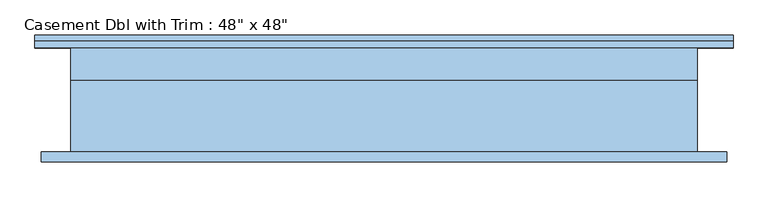
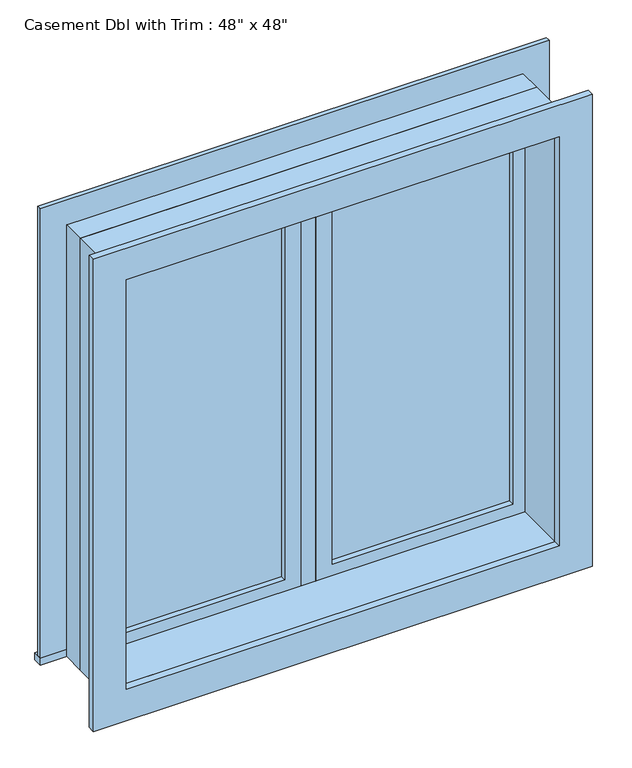
"""IFC4 building model written with IfcOpenShell, lengths in millimetres: window geometry."""

from ifc_helpers import new_model, si_unit, frame, origin, place, context, project, spatial, polyline, outline, extrude, source, transform, mapped, element, save


def window_0862ab64(model_context):
    return source(origin(), model_context, "Body", "SweptSolid", [
        extrude(outline(polyline([(63.5, 85.725), (546.1, 85.725), (546.1, 73.025), (63.5, 73.025), (63.5, 85.725)])), frame((0.0, 0.0, 977.9), z_axis=(0.0, 0.0, 1.0), x_axis=(1.0, 0.0, 0.0)), (0.0, 0.0, 1.0), 1092.2),
        extrude(outline(polyline([(2114.55, 19.05), (933.45, 19.05), (933.45, 590.55), (2114.55, 590.55), (2114.55, 19.05)]), holes=[polyline([(2070.1, 63.5), (2070.1, 546.1), (977.9, 546.1), (977.9, 63.5), (2070.1, 63.5)])]), frame((0.0, 57.15, 0.0), z_axis=(0.0, 1.0, 0.0), x_axis=(0.0, 0.0, 1.0)), (0.0, 0.0, 1.0), 44.45),
        extrude(outline(polyline([(19.05, 57.15), (-19.05, 57.15), (-19.05, 120.65), (19.05, 120.65), (19.05, 57.15)])), frame((0.0, 0.0, 933.45), z_axis=(0.0, 0.0, 1.0), x_axis=(1.0, 0.0, 0.0)), (0.0, 0.0, 1.0), 1181.1),
        extrude(outline(polyline([(-679.45, 146.05), (679.45, 146.05), (679.45, 120.65), (-679.45, 120.65), (-679.45, 146.05)])), frame((0.0, 0.0, 914.4), z_axis=(0.0, 0.0, 1.0), x_axis=(1.0, 0.0, 0.0)), (0.0, 0.0, 1.0), 19.05),
        extrude(outline(polyline([(2114.55, -590.55), (2114.55, 590.55), (933.45, 590.55), (933.45, 679.45), (2203.45, 679.45), (2203.45, -679.45), (933.45, -679.45), (933.45, -590.55), (2114.55, -590.55)])), frame((0.0, 120.65, 0.0), z_axis=(0.0, 1.0, 0.0), x_axis=(0.0, 0.0, 1.0)), (0.0, 0.0, 1.0), 12.7),
        extrude(outline(polyline([(2190.75, 666.75), (2190.75, -666.75), (857.25, -666.75), (857.25, 666.75), (2190.75, 666.75)]), holes=[polyline([(2101.85, 577.85), (946.15, 577.85), (946.15, -577.85), (2101.85, -577.85), (2101.85, 577.85)])]), frame((0.0, -101.6, 0.0), z_axis=(0.0, 1.0, 0.0), x_axis=(0.0, 0.0, 1.0)), (0.0, 0.0, 1.0), 19.05),
        extrude(outline(polyline([(-63.5, 73.025), (-546.1, 73.025), (-546.1, 85.725), (-63.5, 85.725), (-63.5, 73.025)])), frame((0.0, 0.0, 977.9), z_axis=(0.0, 0.0, 1.0), x_axis=(1.0, 0.0, 0.0)), (0.0, 0.0, 1.0), 1092.2),
        extrude(outline(polyline([(2114.55, -590.55), (933.45, -590.55), (933.45, -19.05), (2114.55, -19.05), (2114.55, -590.55)]), holes=[polyline([(2070.1, -546.1), (2070.1, -63.5), (977.9, -63.5), (977.9, -546.1), (2070.1, -546.1)])]), frame((0.0, 57.15, 0.0), z_axis=(0.0, 1.0, 0.0), x_axis=(0.0, 0.0, 1.0)), (0.0, 0.0, 1.0), 44.45),
        extrude(outline(polyline([(2133.6, -609.6), (914.4, -609.6), (914.4, 609.6), (2133.6, 609.6), (2133.6, -609.6)]), holes=[polyline([(2101.85, -577.85), (2101.85, 577.85), (946.15, 577.85), (946.15, -577.85), (2101.85, -577.85)])]), frame((0.0, -82.55, 0.0), z_axis=(0.0, 1.0, 0.0), x_axis=(0.0, 0.0, 1.0)), (0.0, 0.0, 1.0), 139.7),
        extrude(outline(polyline([(2133.6, 609.6), (2133.6, -609.6), (914.4, -609.6), (914.4, 609.6), (2133.6, 609.6)]), holes=[polyline([(2114.55, 590.55), (933.45, 590.55), (933.45, -590.55), (2114.55, -590.55), (2114.55, 590.55)])]), frame((0.0, 57.15, 0.0), z_axis=(0.0, 1.0, 0.0), x_axis=(0.0, 0.0, 1.0)), (0.0, 0.0, 1.0), 63.5),
    ])


if __name__ == "__main__":
    model = new_model("IFC4")
    model_context = context("Model", 3, world=origin())
    ifc_project = project(units=[si_unit("LENGTHUNIT", "METRE", prefix="MILLI")], contexts=[model_context])
    site = spatial("IfcSite", under=ifc_project)
    building = spatial("IfcBuilding", under=site)
    placement = place(None, origin())
    window_shape = window_0862ab64(model_context)
    element("IfcWindow", 1, ObjectType="Casement Dbl with Trim : 48\" x 48\"", at=placement, inside=building, context=model_context, shape_type="MappedRepresentation", body=[
        mapped(window_shape, transform((0.0, 0.0, 0.0), x_axis=(1.0, 0.0, 0.0), y_axis=(0.0, 1.0, 0.0), z_axis=(0.0, 0.0, 1.0))),
    ])
    save(model, "model.ifc")

# Revit data of these elements
# Type "Casement Dbl with Trim : 48\" x 48\""
#   Type Mark = "13"
#   Construction Type Id = "GSP4R"
#   Assembly Code = "B2020100"
#   Analytic Construction = "1/8 in Pilkington single glazing"
#   Visual Light Transmittance = 0.9
#   Thermal Resistance (R) = 1.53941 (h·ft²·°F)/BTU
#   Solar Heat Gain Coefficient = 0.78
#   Heat Transfer Coefficient (U) = 0.6496 BTU/(h·ft²·°F)
#   Height = 4' - 0"
#   Default Sill Height = 3' - 0"
#   Trim Projection - Ext. = 0' - 0 1/2"
#   Trim Projection - Int. = 0' - 0 3/4"
#   Trim Width - Exterior = 0' - 3 1/2"
#   Trim Width - Interior = 0' - 3 1/2"
#   Width = 4' - 0"
#   Window Inset = 0' - 0 3/4"
#   Define Thermal Properties by = 1
#   Glass Pane Material = Glass
#   Sash Material = Sash
#   Trim Exterior Material = Trim
#   Trim Interior Material = Trim
#   Wall Closure = (empty or 0)
# Element 1 (IfcWindow, "Casement Dbl with Trim : 48\" x 48\"")
#   Materials on its faces: "Sash", "Trim", "Glass"
# Materials
#   "Glass": class "Glass", colour RGB 0 128 192, transparency 0.75, Description = "Soda Lime Glass", Cost = 0
#   "Sash": class "Wood", colour RGB 224 178 126, transparency 0
#   "Trim": class "Wood", colour RGB 224 178 126, transparency 0
